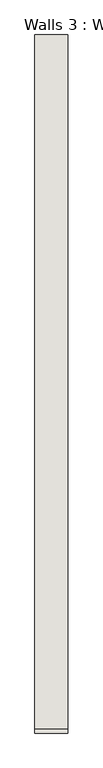
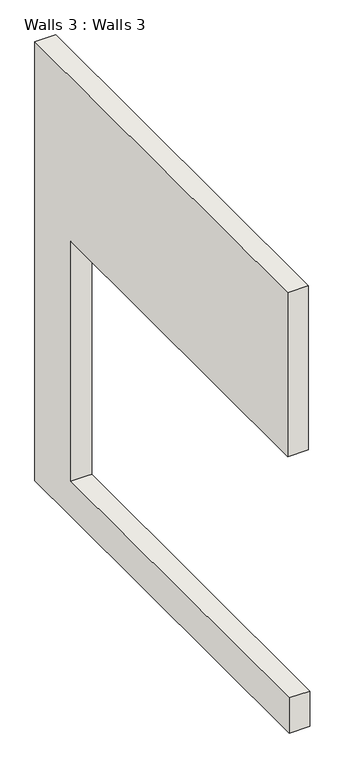
"""IFC4 building model written with IfcOpenShell, lengths in millimetres: wall geometry, Walls 3 : Walls 3."""

from ifc_helpers import new_model, si_unit, frame, origin, place, context, project, spatial, polyline, outline, extrude, source, transform, mapped, element, save


def walls_3_walls_3_a2c954b4(model_context):
    return source(origin(), model_context, "Body", "SweptSolid", [
        extrude(outline(polyline([(270.4399767, 10617.2441528), (6836.8609482, 10617.2441528), (6836.8609482, 7315.2), (6836.8609482, 3657.6), (5902.7435109, 3657.6), (232.3399767, 3657.6), (232.3399767, 4214.183005), (5902.7435109, 4214.183005), (5902.7435109, 8020.2540138), (270.4399767, 8020.2540138), (270.4399767, 10617.2441528)])), frame((-12654.8431118, 0.0, 0.0), z_axis=(1.0, 0.0, 0.0), x_axis=(0.0, 1.0, 0.0)), (0.0, 0.0, 1.0), 309.749841),
    ])


if __name__ == "__main__":
    model = new_model("IFC4")
    model_context = context("Model", 3, world=origin())
    ifc_project = project(units=[si_unit("LENGTHUNIT", "METRE", prefix="MILLI")], contexts=[model_context])
    site = spatial("IfcSite", under=ifc_project)
    building = spatial("IfcBuilding", under=site)
    placement = place(None, origin())
    walls_3_walls_3_shape = walls_3_walls_3_a2c954b4(model_context)
    element("IfcWall", 1, ObjectType="Walls 3 : Walls 3", at=placement, inside=building, context=model_context, shape_type="MappedRepresentation", body=[
        mapped(walls_3_walls_3_shape, transform((0.0, 0.0, 0.0), x_axis=(1.0, 0.0, 0.0), y_axis=(0.0, 1.0, 0.0), z_axis=(0.0, 0.0, 1.0))),
    ])
    save(model, "model.ifc")

# Revit data of these elements
# Element 1 (IfcWall, "Walls 3 : Walls 3")
#   Materials on its faces: "Default Wall"
# Materials
#   "Default Wall": colour RGB 128 128 128, transparency 0
